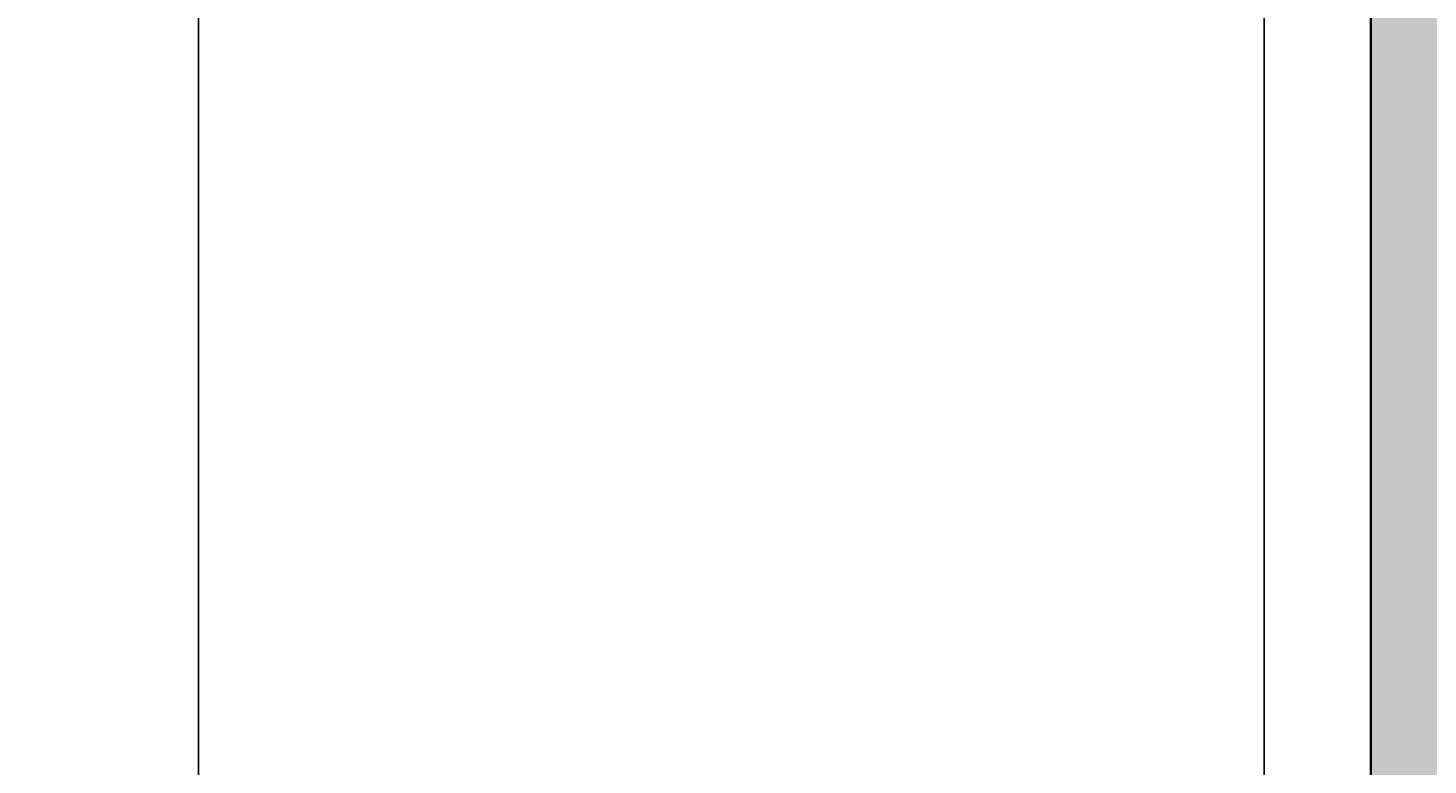
# Model space of a CAD drawing. Units: inches. Extents: x 1998 to 2588, y 1139 to 1977.
# Tile 26 of 134: x 2289 to 2344, y 1427 to 1456. Entities that reach past the tile are written whole.
import ezdxf

# ---------------------------------------------------------------- set-up
doc = ezdxf.new("R2010")
doc.units = ezdxf.units.IN
for name, color, linetype, lineweight in [('A-ANNO-DIMS', 2, 'Continuous', 18), ('A-WALL-PATT', 252, 'Continuous', 13), ('WALL', 200, 'Continuous', 35)]:
    doc.layers.add(name, color=color, linetype=linetype, lineweight=lineweight)
doc.styles.get("Standard").update_dxf_attribs({"font": 'arial.ttf'})
doc.dimstyles.get("Standard").update_dxf_attribs({"dimtxt": 0.18, "dimasz": 0.18, "dimexe": 0.18, "dimexo": 0.0625, "dimgap": 0.09, "dimtad": 0, "dimtih": 1, "dimtoh": 1, "dimdec": 4, "dimzin": 0, "dimdsep": 46, "dimtxsty": 'Standard', "dimcen": 0.09, "dimadec": 0, "dimazin": 0, "dimtfac": 1, "dimtdec": 4, "dimtofl": 0, "dimtmove": 0, "dimatfit": 3, "dimfxl": 1, "dimtolj": 1, "dimtzin": 0, "dimarcsym": 0})

# ---------------------------------------------------------------- blocks, each defined once
blk = doc.blocks.new('*D23')
at = {"layer": 'A-ANNO-DIMS', "color": 0, "lineweight": -2, "transparency": 16777216}
for p, q in [((2549.179, 1476.17), (2549.179, 1138.602)), ((2059.473, 1413.17), (2059.473, 1138.602)), ((2059.653, 1138.782), (2303.928, 1138.782)), ((2548.999, 1138.782), (2304.723, 1138.782))]:
    blk.add_line(p, q, dxfattribs=at)
at = {"layer": 'A-ANNO-DIMS', "color": 0, "transparency": 16777216}
for points in [[(2059.653, 1138.812), (2059.653, 1138.752), (2059.473, 1138.782)], [(2548.999, 1138.812), (2548.999, 1138.752), (2549.179, 1138.782)]]:
    blk.add_solid(points, dxfattribs=at)
at = {"layer": 'Defpoints', "color": 0, "transparency": 16777216}
for p in [(2549.179, 1476.232), (2059.473, 1413.232), (2549.179, 1138.782)]:
    blk.add_point(p, dxfattribs=at)
at = {"layer": 'A-ANNO-DIMS', "color": 0, "transparency": 16777216, "insert": (2304.326, 1138.782), "char_height": 0.18, "attachment_point": 5}
blk.add_mtext('\\A1;489.7', dxfattribs=at)
blk = doc.blocks.new('*D44')
at = {"layer": 'A-ANNO-DIMS', "color": 0, "lineweight": -2, "transparency": 16777216}
for p, q in [((2295.414, 1588.67), (2295.414, 1138.602)), ((2337.287, 1588.67), (2337.287, 1138.602)), ((2295.594, 1138.782), (2315.953, 1138.782)), ((2337.107, 1138.782), (2316.748, 1138.782))]:
    blk.add_line(p, q, dxfattribs=at)
at = {"layer": 'A-ANNO-DIMS', "color": 0, "transparency": 16777216}
for points in [[(2295.594, 1138.812), (2295.594, 1138.752), (2295.414, 1138.782)], [(2337.107, 1138.812), (2337.107, 1138.752), (2337.287, 1138.782)]]:
    blk.add_solid(points, dxfattribs=at)
at = {"layer": 'Defpoints', "color": 0, "transparency": 16777216}
for p in [(2295.414, 1588.732), (2337.287, 1588.732), (2337.287, 1138.782)]:
    blk.add_point(p, dxfattribs=at)
at = {"layer": 'A-ANNO-DIMS', "color": 0, "transparency": 16777216, "insert": (2316.35, 1138.782), "char_height": 0.18, "attachment_point": 5}
blk.add_mtext('\\A1;41.87', dxfattribs=at)

msp = doc.modelspace()

# ---------------------------------------------------------------- hatches: boundary and pattern name
at = {"layer": 'A-WALL-PATT'}
h = msp.add_hatch(color=256, dxfattribs=at)
h.dxf.hatch_style = 1
h.paths.add_polyline_path([(2222.9729, 1888.7324), (2099.4125, 1888.7324), (2099.4125, 1879.7324), (2222.9729, 1879.7324)])
h.paths.add_polyline_path([(2096.9729, 1868.3278), (2087.9729, 1868.3278), (2087.9729, 1775.637), (2096.9729, 1775.637)])
h.paths.add_polyline_path([(2227.4729, 1868.3278), (2222.9729, 1868.3278), (2222.9729, 1774.3318), (2227.4729, 1774.3318)])
h.paths.add_polyline_path([(2188.3019, 1759.7324), (2138.6074, 1759.7324), (2099.4125, 1759.7324), (2099.4125, 1755.2324), (2176.9729, 1755.2324), (2188.3019, 1755.2324)])
h.paths.add_polyline_path([(2087.9729, 1759.7324), (2059.4729, 1759.7324), (2059.4729, 1702.7324), (2087.9729, 1702.7324), (2087.9729, 1707.2324), (2063.9729, 1707.2324), (2063.9729, 1755.2324), (2087.9729, 1755.2324)])
h.paths.add_polyline_path([(2096.9729, 1755.2324), (2087.9729, 1755.2324), (2087.9729, 1707.2324), (2096.9729, 1707.2324)])
h.paths.add_polyline_path([(2187.0461, 1707.2324), (2105.9729, 1707.2324), (2096.9729, 1707.2324), (2087.9729, 1707.2324), (2087.9729, 1702.7324), (2105.9729, 1702.7324), (2114.9729, 1702.7324), (2187.0461, 1702.7324)])
h.paths.add_polyline_path([(2181.4729, 1719.2028), (2176.9729, 1719.2028), (2176.9729, 1707.2324), (2181.4729, 1707.2324)])
h.paths.add_polyline_path([(2216.0332, 1588.7324), (2114.9729, 1588.7324), (2105.9729, 1588.7324), (2105.9729, 1584.2324), (2216.0332, 1584.2324)])
h.paths.add_polyline_path([(2077.691, 1588.7324), (2061.4729, 1588.7324), (2061.4729, 1584.2324), (2077.691, 1584.2324)])
h.paths.add_polyline_path([(2105.9729, 1588.7324), (2098.0956, 1588.7324), (2098.0956, 1584.2324), (2105.9729, 1584.2324)])
h.paths.add_polyline_path([(2114.9729, 1596.2642), (2110.1012, 1596.2642), (2105.9729, 1596.2642), (2105.9729, 1588.7324), (2114.9729, 1588.7324)])
h.paths.add_polyline_path([(2114.9729, 1584.2324), (2105.9729, 1584.2324), (2105.9729, 1580.249), (2110.1012, 1580.249), (2114.9729, 1580.249)])
h.paths.add_polyline_path([(2114.9729, 1547.7716), (2110.1012, 1547.7716, -0.0318759), (2105.9729, 1548.035), (2105.9729, 1470.2324), (2108.3775, 1470.2324), (2108.3775, 1465.7324), (2186.2943, 1465.7324), (2186.2943, 1470.2324), (2114.9729, 1470.2324)])
h.paths.add_polyline_path([(2227.4729, 1584.2324), (2222.9729, 1584.2324), (2222.9729, 1486.137), (2227.4729, 1486.137)])
h.paths.add_polyline_path([(2295.4138, 1593.2324), (2227.4729, 1593.2324), (2227.4729, 1588.7324), (2295.4138, 1588.7324), (2295.4138, 1591.8729)])
h.paths.add_polyline_path([(2345.9729, 1627.1165), (2341.4729, 1627.1165), (2341.4729, 1593.2324), (2337.2869, 1593.2324), (2337.2869, 1591.8729), (2337.2869, 1588.7324), (2345.9729, 1588.7324)])
h.paths.add_polyline_path([(2291.9729, 1588.7324), (2287.4729, 1588.7324), (2287.4729, 1522.7324), (2291.9729, 1522.7324)])
h.paths.add_polyline_path([(2291.9729, 1522.7324), (2287.4729, 1522.7324), (2227.4729, 1522.7324), (2227.4729, 1518.2324), (2291.9729, 1518.2324)])
h.paths.add_polyline_path([(2295.7347, 1519.5919), (2295.7347, 1522.7324), (2291.9729, 1522.7324), (2291.9729, 1518.2324), (2295.7347, 1518.2324)])
h.paths.add_polyline_path([(2345.9729, 1522.7324), (2337.6078, 1522.7324), (2337.6078, 1519.5919), (2337.6078, 1518.2324), (2341.4729, 1518.2324), (2341.4729, 1488.5616), (2345.9729, 1488.5616)])
h.paths.add_polyline_path([(2345.9729, 1468.1569), (2341.4729, 1468.1569), (2341.4729, 1374.2324), (2227.4729, 1374.2324), (2227.4729, 1369.7324), (2345.9729, 1369.7324)])
h.paths.add_polyline_path([(2345.9729, 1369.7324), (2341.4729, 1369.7324), (2341.4729, 1362.2324), (2345.9729, 1362.2324)])
h.paths.add_polyline_path([(2345.9729, 1317.7324), (2345.9729, 1322.2324), (2341.4729, 1322.2324), (2341.4729, 1285.137), (2345.9729, 1285.137)], flags=17)
h.paths.add_polyline_path([(2356.2096, 1322.2324), (2345.9729, 1322.2324), (2345.9729, 1317.7324), (2356.2096, 1317.7324), (2356.2096, 1319.3088)], flags=17)
h.paths.add_polyline_path([(2393.9729, 1322.2324), (2375.6999, 1322.2324), (2375.6999, 1319.3088, -0.0202458), (2375.636, 1317.7324), (2393.9729, 1317.7324)], flags=17)
h.paths.add_polyline_path([(2398.4729, 1322.2324), (2393.9729, 1322.2324), (2393.9729, 1317.7324), (2393.9729, 1237.7324), (2345.9729, 1237.7324), (2345.9729, 1264.7324), (2341.4729, 1264.7324), (2341.4729, 1228.7324), (2393.9729, 1228.7324), (2482.7412, 1228.7324), (2482.7412, 1237.7324), (2398.4729, 1237.7324), (2398.4729, 1297.1029)])
h.paths.add_polyline_path([(2398.4729, 1362.2324), (2393.9729, 1362.2324), (2393.9729, 1357.7324), (2398.4729, 1357.7324)])
h.paths.add_polyline_path([(2345.9729, 1329.7549), (2341.4729, 1329.7549), (2341.4729, 1322.2324), (2345.9729, 1322.2324)])

# ---------------------------------------------------------------- linework, layer by layer
at = {"layer": 'WALL'}
msp.add_line((2341.4729, 1468.1569), (2341.4729, 1374.2324), dxfattribs=at)

# ---------------------------------------------------------------- dimensions: what is measured, and where the dimension line sits
at = {"layer": 'A-ANNO-DIMS'}
for base, p1, p2, override, picture, middle in [((2337.2869, 1138.7824), (2295.4138, 1588.7324), (2337.2869, 1588.7324), {"dimdec": 2, "dimlfac": 1, "dimrnd": 0, "dimzin": 0, "dimdsep": 46, "dimlunit": 2}, '*D44', (2316.3503, 1138.7824)), ((2549.1786, 1138.7824), (2059.4729, 1413.2324), (2549.1786, 1476.2324), {"dimdec": 1, "dimlfac": 1, "dimrnd": 0, "dimzin": 0, "dimdsep": 46, "dimlunit": 2}, '*D23', (2304.3257, 1138.7824))]:
    dim = msp.add_linear_dim(base=base, p1=p1, p2=p2, dimstyle='Standard', override=override, dxfattribs=at)
    dim.commit()
    dim.dimension.update_dxf_attribs({"geometry": picture, "text_midpoint": middle})

doc.saveas('drawing.dxf')
